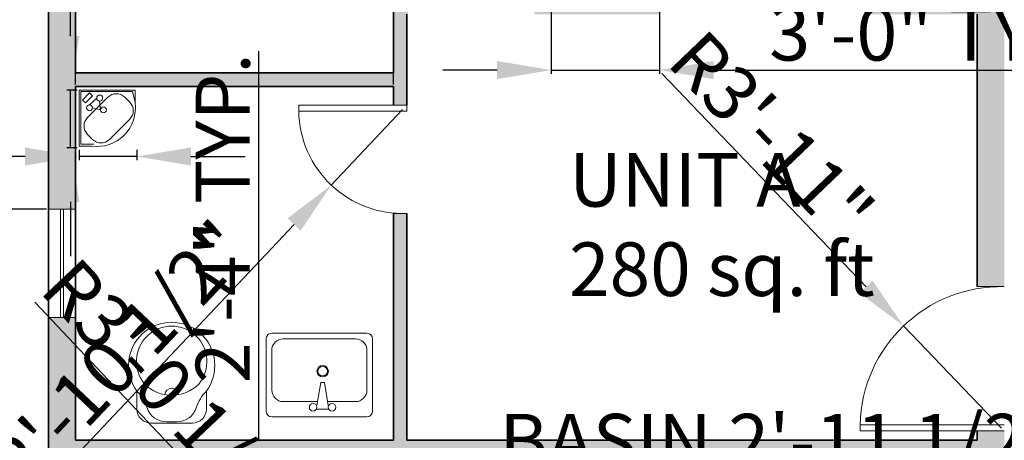
# Model space of a CAD drawing. Units: inches. Extents: x 2043 to 3177, y 1429 to 2563.
# Tile 10 of 14: x 2224 to 2552, y 1952 to 2092. Entities that reach past the tile are written whole.
import ezdxf

# ---------------------------------------------------------------- set-up
doc = ezdxf.new("R2010")
doc.units = ezdxf.units.IN
for name, color, linetype, lineweight in [('A-ANNO-DIMS', 2, 'Continuous', 13), ('A-AREA-IDEN', 7, 'Continuous', 18), ('A-DOOR', 3, 'Continuous', 18), ('A-FLOR-FIXT', 8, 'Continuous', 18), ('A-GLAZ', 4, 'Continuous', 18), ('A-WALL', 7, 'Continuous', 35)]:
    doc.layers.add(name, color=color, linetype=linetype, lineweight=lineweight)
doc.layers.add('A-WALL-PATT', color=251, linetype='Continuous', lineweight=13, true_color=0x636466)
doc.styles.add('DIM_FONT', font='TXT.shx', dxfattribs={"width": 0.8})
doc.styles.get("Standard").update_dxf_attribs({"font": 'arial.ttf'})
doc.dimstyles.new('ISO-25', dxfattribs={"dimtxt": 18, "dimasz": 18, "dimexe": 1.25, "dimexo": 0.625, "dimtad": 1, "dimlunit": 3, "dimtxsty": 'Standard', "dimcen": 2.5, "dimadec": 0, "dimazin": 0, "dimtfac": 1, "dimtmove": 0, "dimatfit": 3, "dimfxl": 1, "dimarcsym": 0})

# ---------------------------------------------------------------- blocks, each defined once
blk = doc.blocks.new('A$C6EF51710')
at = {"linetype": 'ByBlock'}
for p, q in [((0.0508, 0.2843), (0.1169, 0.2843)), ((0, 0.0811), (0, 0.2335)), ((0.0041, 0.1392), (0.0041, 0.1755)), ((0.1169, 0.0303), (0.0508, 0.0303))]:
    blk.add_line(p, q, dxfattribs=at)
for centre, radius, start, end in [((0.2107, 0.1573), 0.1576, 232.8984, 127.1016), ((0.0508, 0.2335), 0.0508, 90, 180), ((0.0168, 0.3818), 0.1397, 287.1046, 315), ((0.2413, 0.1573), 0.1397, 135, 225), ((0.2254, 0.1573), 0.1289, 230.0084, 129.9916), ((0.0803, 0.1755), 0.0762, 107.1046, 180), ((0.1016, 0.1573), 0.0254, 275.2159, 84.7841), ((0.0803, 0.1392), 0.0762, 180, 252.8954), ((0.0508, 0.0811), 0.0508, 180, 270), ((0.0168, -0.0672), 0.1397, 45, 72.8954)]:
    blk.add_arc(centre, radius, start, end, dxfattribs=at)
blk = doc.blocks.new('A$C03A44EBA')
at = {"rotation": 270}
blk.add_blockref('A$C6EF51710', (0.0003, 0.3683), dxfattribs=at)
blk = doc.blocks.new('A$C564A496C')
at = {"linetype": 'ByBlock'}
for p, q in [((543.2, 450), (30.7, 450)), ((0, 419.3), (0, 30.7)), ((238.5, 409.1), (299.8, 409.1)), ((238.5, 388.6), (258.9, 265.9)), ((279.4, 265.9), (299.8, 388.6)), ((573.8, 30.7), (573.8, 419.3)), ((92, 368.2), (243.6, 368.2)), ((294.7, 368.2), (481.8, 368.2)), ((30.7, 92), (30.7, 306.8)), ((258.9, 265.9), (279.4, 265.9)), ((543.2, 306.8), (543.2, 92)), ((30.7, 0), (543.2, 0)), ((481.8, 30.7), (92, 30.7))]:
    blk.add_line(p, q, dxfattribs=at)
for centre, radius in [((218, 398.9), 20.5), ((320.3, 398.9), 20.5), ((269.1, 204.5), 30.7), ((269.1, 204.5), 25.7)]:
    blk.add_circle(centre, radius, dxfattribs=at)
for centre, radius, start, end in [((30.7, 419.3), 30.7, 90, 180), ((543.2, 419.3), 30.7, 0, 90), ((92, 306.8), 61.4, 90, 180), ((481.8, 306.8), 61.4, 0, 90), ((92, 92), 61.4, 180, 270), ((481.8, 92), 61.4, 270, 0), ((30.7, 30.7), 30.7, 180, 270), ((543.2, 30.7), 30.7, 270, 0)]:
    blk.add_arc(centre, radius, start, end, dxfattribs=at)
at = {"style": 'DIM_FONT', "width": 0.8, "flags": 9}
for tag in ['YSIZE', 'XSIZE']:
    blk.add_attdef(tag, (269.1, 450), '', height=0.5, rotation=270, dxfattribs=at)
blk = doc.blocks.new('A$C017A17F4')
for p, q in [((0.45, 0.45), (0, 0.45)), ((0, 0.45), (0, 0.35)), ((0.3467, 0.3997), (0.3704, 0.4234)), ((0.4041, 0.3423), (0.3467, 0.3997)), ((0.3704, 0.4234), (0.4278, 0.366)), ((0.45, 0), (0.45, 0.45)), ((0.0533, 0.3414), (0.094, 0.3821)), ((0.2297, 0.3821), (0.3933, 0.2185)), ((0.4278, 0.366), (0.4041, 0.3423)), ((0.2168, 0.0421), (0.0533, 0.2056)), ((0.3933, 0.0827), (0.3526, 0.0421)), ((0.35, 0), (0.45, 0))]:
    blk.add_line(p, q)
at = {"ltscale": 10}
for p, q in [((0.4392, 0.4359), (0.0144, 0.4359)), ((0.0144, 0.4359), (0.0144, 0.3323)), ((0.4392, 0.4359), (0.4392, 0.0216)), ((0.3078, 0.342), (0.2911, 0.2778)), ((0.3317, 0.3659), (0.3861, 0.3086)), ((0.3622, 0.2847), (0.2911, 0.2778)), ((0.4392, 0.0216), (0.35, 0))]:
    blk.add_line(p, q, dxfattribs=at)
for centre in [(0.3078, 0.3659), (0.2911, 0.2539), (0.3861, 0.2847)]:
    blk.add_circle(centre, 0.0239, dxfattribs=at)
for centre, radius, start, end in [((0.1618, 0.3142), 0.096, 45, 135), ((0.3045, 0.3045), 0.3079, 171.50989, 278.49011), ((0.1212, 0.2735), 0.096, 135, 225), ((0.3254, 0.1506), 0.096, 315, 45), ((0.2847, 0.11), 0.096, 225, 315)]:
    blk.add_arc(centre, radius, start, end)
blk = doc.blocks.new('*D26')
at = {"layer": 'A-ANNO-DIMS', "color": 0, "lineweight": -2, "transparency": 16777216}
for p, q in [((2233.12, 2029.27), (2166.79, 2029.27)), ((2168.04, 1902.52), (2168.04, 2011.27)), ((2233.12, 1884.52), (2166.79, 1884.52))]:
    blk.add_line(p, q, dxfattribs=at)
at = {"layer": 'A-ANNO-DIMS', "color": 0, "transparency": 16777216}
for points in [[(2165.04, 2011.27), (2171.04, 2011.27), (2168.04, 2029.27)], [(2165.04, 1902.52), (2171.04, 1902.52), (2168.04, 1884.52)]]:
    blk.add_solid(points, dxfattribs=at)
at = {"layer": 'Defpoints', "color": 0, "transparency": 16777216}
for p in [(2168.04, 2029.27), (2233.74, 2029.27), (2233.74, 1884.52)]:
    blk.add_point(p, dxfattribs=at)
at = {"layer": 'A-ANNO-DIMS', "color": 0, "transparency": 16777216, "insert": (2158.23, 1956.89), "char_height": 18, "attachment_point": 5, "rotation": 90}
blk.add_mtext('19\'-0"', dxfattribs=at)
blk = doc.blocks.new('*D27')
at = {"layer": 'A-ANNO-DIMS', "color": 0, "lineweight": -2, "transparency": 16777216}
for p, q in [((2233.12, 2261.39), (2165.87, 2261.39)), ((2167.12, 2047.27), (2167.12, 2243.39)), ((2233.12, 2029.27), (2165.87, 2029.27))]:
    blk.add_line(p, q, dxfattribs=at)
at = {"layer": 'A-ANNO-DIMS', "color": 0, "transparency": 16777216}
for points in [[(2164.12, 2243.39), (2170.12, 2243.39), (2167.12, 2261.39)], [(2164.12, 2047.27), (2170.12, 2047.27), (2167.12, 2029.27)]]:
    blk.add_solid(points, dxfattribs=at)
at = {"layer": 'Defpoints', "color": 0, "transparency": 16777216}
for p in [(2167.12, 2261.39), (2233.74, 2261.39), (2233.74, 2029.27)]:
    blk.add_point(p, dxfattribs=at)
at = {"layer": 'A-ANNO-DIMS', "color": 0, "transparency": 16777216, "insert": (2157.3, 2145.33), "char_height": 18, "attachment_point": 5, "rotation": 90}
blk.add_mtext('25\'-0"', dxfattribs=at)
blk = doc.blocks.new('*D28')
at = {"layer": 'A-ANNO-DIMS', "color": 0, "lineweight": -2, "transparency": 16777216}
for p, q in [((2233.12, 2261.39), (2064.1, 2261.39)), ((2065.35, 2243.39), (2065.35, 1652.39)), ((2233.12, 1634.39), (2064.1, 1634.39))]:
    blk.add_line(p, q, dxfattribs=at)
at = {"layer": 'A-ANNO-DIMS', "color": 0, "transparency": 16777216}
for points in [[(2062.35, 2243.39), (2068.35, 2243.39), (2065.35, 2261.39)], [(2062.35, 1652.39), (2068.35, 1652.39), (2065.35, 1634.39)]]:
    blk.add_solid(points, dxfattribs=at)
at = {"layer": 'Defpoints', "color": 0, "transparency": 16777216}
for p in [(2233.74, 2261.39), (2065.35, 1634.39), (2233.74, 1634.39)]:
    blk.add_point(p, dxfattribs=at)
at = {"layer": 'A-ANNO-DIMS', "color": 0, "transparency": 16777216, "insert": (2055.54, 1947.89), "char_height": 18, "attachment_point": 5, "rotation": 90}
blk.add_mtext('75\'-0"', dxfattribs=at)
blk = doc.blocks.new('GLAZING-36')
for p, q in [((0, 36), (0, 0)), ((1, 36), (1, 0))]:
    blk.add_line(p, q)
blk = doc.blocks.new('*D57')
at = {"layer": 'A-ANNO-DIMS', "color": 0, "lineweight": -2, "transparency": 16777216}
for p, q in [((2291.03, 1939.93), (2273.03, 1939.93)), ((2309.03, 1935.24), (2309.03, 1941.18)), ((2309.03, 1939.93), (2344.46, 1939.93)), ((2344.46, 1935.24), (2344.46, 1941.18)), ((2362.46, 1939.93), (2629.01, 1939.93))]:
    blk.add_line(p, q, dxfattribs=at)
at = {"layer": 'A-ANNO-DIMS', "color": 0, "transparency": 16777216}
for points in [[(2291.03, 1942.93), (2291.03, 1936.93), (2309.03, 1939.93)], [(2362.46, 1942.93), (2362.46, 1936.93), (2344.46, 1939.93)]]:
    blk.add_solid(points, dxfattribs=at)
at = {"layer": 'Defpoints', "color": 0, "transparency": 16777216}
for p in [(2344.46, 1939.93), (2309.03, 1934.62), (2344.46, 1934.62)]:
    blk.add_point(p, dxfattribs=at)
at = {"layer": 'A-ANNO-DIMS', "color": 0, "transparency": 16777216, "insert": (2504.74, 1949.86), "char_height": 18, "attachment_point": 5}
blk.add_mtext('BASIN 2\'-11 1/2" TYP.', dxfattribs=at)
blk = doc.blocks.new('*D58')
at = {"layer": 'A-ANNO-DIMS', "color": 0, "lineweight": -2, "transparency": 16777216}
for p, q in [((2303.72, 1952.62), (2303.72, 2081.89)), ((2308.41, 1934.62), (2302.47, 1934.62)), ((2303.72, 1906.83), (2303.72, 1934.62)), ((2308.41, 1906.83), (2302.47, 1906.83)), ((2303.72, 1888.83), (2303.72, 1870.83))]:
    blk.add_line(p, q, dxfattribs=at)
at = {"layer": 'A-ANNO-DIMS', "color": 0, "transparency": 16777216}
for points in [[(2300.72, 1952.62), (2306.72, 1952.62), (2303.72, 1934.62)], [(2300.72, 1888.83), (2306.72, 1888.83), (2303.72, 1906.83)]]:
    blk.add_solid(points, dxfattribs=at)
at = {"layer": 'Defpoints', "color": 0, "transparency": 16777216}
for p in [(2303.72, 1934.62), (2309.03, 1934.62), (2309.03, 1906.83)]:
    blk.add_point(p, dxfattribs=at)
at = {"layer": 'A-ANNO-DIMS', "color": 0, "transparency": 16777216, "insert": (2294.05, 2026.26), "char_height": 18, "attachment_point": 5, "rotation": 90}
blk.add_mtext('2\'-4" TYP.', dxfattribs=at)
blk = doc.blocks.new('*D59')
at = {"layer": 'A-ANNO-DIMS', "color": 0, "lineweight": -2, "transparency": 16777216}
for p, q in [((2241.04, 2086.9), (2241.04, 2414.07)), ((2243.29, 2068.9), (2239.79, 2068.9)), ((2241.04, 2049.7), (2241.04, 2068.9)), ((2243.29, 2049.7), (2239.79, 2049.7)), ((2241.04, 2031.7), (2241.04, 2013.7))]:
    blk.add_line(p, q, dxfattribs=at)
at = {"layer": 'A-ANNO-DIMS', "color": 0, "transparency": 16777216}
for points in [[(2238.04, 2086.9), (2244.04, 2086.9), (2241.04, 2068.9)], [(2238.04, 2031.7), (2244.04, 2031.7), (2241.04, 2049.7)]]:
    blk.add_solid(points, dxfattribs=at)
at = {"layer": 'Defpoints', "color": 0, "transparency": 16777216}
for p in [(2241.04, 2068.9), (2243.92, 2068.9), (2243.92, 2049.7)]:
    blk.add_point(p, dxfattribs=at)
at = {"layer": 'A-ANNO-DIMS', "color": 0, "transparency": 16777216, "insert": (2231.1, 2259.48), "char_height": 18, "attachment_point": 5, "rotation": 90}
blk.add_mtext('CORNER BASIN 1\'-7" TYP.', dxfattribs=at)
blk = doc.blocks.new('*D60')
at = {"layer": 'A-ANNO-DIMS', "color": 0, "lineweight": -2, "transparency": 16777216}
for p, q in [((2243.92, 2049.08), (2243.92, 2045.57)), ((2263.12, 2049.08), (2263.12, 2045.57)), ((2225.92, 2046.82), (2098.64, 2046.82)), ((2263.12, 2046.82), (2243.92, 2046.82)), ((2281.12, 2046.82), (2299.12, 2046.82))]:
    blk.add_line(p, q, dxfattribs=at)
at = {"layer": 'A-ANNO-DIMS', "color": 0, "transparency": 16777216}
for points in [[(2225.92, 2049.82), (2225.92, 2043.82), (2243.92, 2046.82)], [(2281.12, 2049.82), (2281.12, 2043.82), (2263.12, 2046.82)]]:
    blk.add_solid(points, dxfattribs=at)
at = {"layer": 'Defpoints', "color": 0, "transparency": 16777216}
for p in [(2243.92, 2049.7), (2263.12, 2049.7), (2243.92, 2046.82)]:
    blk.add_point(p, dxfattribs=at)
at = {"layer": 'A-ANNO-DIMS', "color": 0, "transparency": 16777216, "insert": (2153.28, 2056.49), "char_height": 18, "attachment_point": 5}
blk.add_mtext('1\'-7" TYP.', dxfattribs=at)
blk = doc.blocks.new('*D61')
at = {"layer": 'A-ANNO-DIMS', "color": 0, "lineweight": -2, "transparency": 16777216}
for p, q in [((2752.39, 1913.46), (2434.98, 1913.46)), ((2770.39, 1916.38), (2770.39, 1912.21)), ((2794.01, 1913.46), (2770.39, 1913.46)), ((2794.01, 1916.38), (2794.01, 1912.21)), ((2812.01, 1913.46), (2830.01, 1913.46))]:
    blk.add_line(p, q, dxfattribs=at)
at = {"layer": 'A-ANNO-DIMS', "color": 0, "transparency": 16777216}
for points in [[(2752.39, 1916.46), (2752.39, 1910.46), (2770.39, 1913.46)], [(2812.01, 1916.46), (2812.01, 1910.46), (2794.01, 1913.46)]]:
    blk.add_solid(points, dxfattribs=at)
at = {"layer": 'Defpoints', "color": 0, "transparency": 16777216}
for p in [(2770.39, 1917.01), (2794.01, 1917.01), (2770.39, 1913.46)]:
    blk.add_point(p, dxfattribs=at)
at = {"layer": 'A-ANNO-DIMS', "color": 0, "transparency": 16777216, "insert": (2584.68, 1923.4), "char_height": 18, "attachment_point": 5}
blk.add_mtext('COOKTOP 1\'-11 1/2" TYP.', dxfattribs=at)
blk = doc.blocks.new('*D64')
at = {"layer": 'A-ANNO-DIMS', "color": 0, "lineweight": -2, "transparency": 16777216}
for p, q in [((2400.99, 2098.02), (2400.99, 2074.33)), ((2436.99, 2098.02), (2436.99, 2074.33)), ((2382.99, 2075.58), (2364.99, 2075.58)), ((2400.99, 2075.58), (2436.99, 2075.58)), ((2454.99, 2075.58), (2583.95, 2075.58))]:
    blk.add_line(p, q, dxfattribs=at)
at = {"layer": 'A-ANNO-DIMS', "color": 0, "transparency": 16777216}
for points in [[(2382.99, 2078.58), (2382.99, 2072.58), (2400.99, 2075.58)], [(2454.99, 2078.58), (2454.99, 2072.58), (2436.99, 2075.58)]]:
    blk.add_solid(points, dxfattribs=at)
at = {"layer": 'Defpoints', "color": 0, "transparency": 16777216}
for p in [(2400.99, 2098.64), (2436.99, 2098.64), (2436.99, 2075.58)]:
    blk.add_point(p, dxfattribs=at)
at = {"layer": 'A-ANNO-DIMS', "color": 0, "transparency": 16777216, "insert": (2528.47, 2085.4), "char_height": 18, "attachment_point": 5}
blk.add_mtext('3\'-0" TYP.', dxfattribs=at)
blk = doc.blocks.new('*D73')
at = {"layer": 'A-ANNO-DIMS', "color": 0, "lineweight": -2, "transparency": 16777216}
for p, q in [((2242.74, 2070.77), (2242.74, 2125.49)), ((2260.74, 2124.24), (2330.49, 2124.24)), ((2348.49, 2070.77), (2348.49, 2125.49))]:
    blk.add_line(p, q, dxfattribs=at)
at = {"layer": 'A-ANNO-DIMS', "color": 0, "transparency": 16777216}
for points in [[(2260.74, 2127.24), (2260.74, 2121.24), (2242.74, 2124.24)], [(2330.49, 2127.24), (2330.49, 2121.24), (2348.49, 2124.24)]]:
    blk.add_solid(points, dxfattribs=at)
at = {"layer": 'Defpoints', "color": 0, "transparency": 16777216}
for p in [(2348.49, 2124.24), (2242.74, 2070.14), (2348.49, 2070.14)]:
    blk.add_point(p, dxfattribs=at)
at = {"layer": 'A-ANNO-DIMS', "color": 0, "transparency": 16777216, "insert": (2295.62, 2134.06), "char_height": 18, "attachment_point": 5}
blk.add_mtext('8\'-10"', dxfattribs=at)
blk = doc.blocks.new('*D83')
at = {"layer": 'A-ANNO-DIMS', "color": 0, "lineweight": -2, "transparency": 16777216}
for p, q in [((2437.75, 2074.42), (2505.77, 2003.44)), ((2550.78, 1956.48), (2518.23, 1990.44))]:
    blk.add_line(p, q, dxfattribs=at)
at = {"layer": 'A-ANNO-DIMS', "color": 0, "transparency": 16777216}
blk.add_solid([(2507.94, 2005.52), (2503.61, 2001.36), (2518.23, 1990.44)], dxfattribs=at)
at = {"layer": 'Defpoints', "color": 0, "transparency": 16777216}
for p in [(2518.23, 1990.44), (2550.78, 1956.48)]:
    blk.add_point(p, dxfattribs=at)
at = {"layer": 'A-ANNO-DIMS', "color": 0, "transparency": 16777216, "insert": (2472.63, 2052.22), "char_height": 18, "attachment_point": 5, "rotation": 313.7813}
blk.add_mtext('R3\'-11"', dxfattribs=at)
blk = doc.blocks.new('*D91')
at = {"layer": 'A-ANNO-DIMS', "color": 0, "lineweight": -2, "transparency": 16777216}
for p, q in [((2229.24, 1998.38), (2315.93, 1906.58)), ((2353.2, 1867.12), (2328.29, 1893.49))]:
    blk.add_line(p, q, dxfattribs=at)
at = {"layer": 'A-ANNO-DIMS', "color": 0, "transparency": 16777216}
blk.add_solid([(2318.11, 1908.64), (2313.75, 1904.52), (2328.29, 1893.49)], dxfattribs=at)
at = {"layer": 'Defpoints', "color": 0, "transparency": 16777216}
for p in [(2328.29, 1893.49), (2353.2, 1867.12)]:
    blk.add_point(p, dxfattribs=at)
at = {"layer": 'A-ANNO-DIMS', "color": 0, "transparency": 16777216, "insert": (2273.63, 1965.84), "char_height": 18, "attachment_point": 5, "rotation": 313.3628}
blk.add_mtext('R3\'-0 1/2"', dxfattribs=at)
blk = doc.blocks.new('*D92')
at = {"layer": 'A-ANNO-DIMS', "color": 0, "lineweight": -2, "transparency": 16777216}
for p, q in [((2351.56, 2062.42), (2327.82, 2037.29)), ((2219.16, 1922.24), (2315.46, 2024.21))]:
    blk.add_line(p, q, dxfattribs=at)
at = {"layer": 'A-ANNO-DIMS', "color": 0, "transparency": 16777216}
blk.add_solid([(2313.28, 2026.27), (2317.64, 2022.15), (2327.82, 2037.29)], dxfattribs=at)
at = {"layer": 'Defpoints', "color": 0, "transparency": 16777216}
for p in [(2351.56, 2062.42), (2327.82, 2037.29)]:
    blk.add_point(p, dxfattribs=at)
at = {"layer": 'A-ANNO-DIMS', "color": 0, "transparency": 16777216, "insert": (2253.91, 1973.5), "char_height": 18, "attachment_point": 5, "rotation": 46.6358}
blk.add_mtext('R2\'-10 1/2"', dxfattribs=at)

msp = doc.modelspace()

# ---------------------------------------------------------------- hatches: boundary and pattern name
at = {"layer": 'A-WALL-PATT'}
h = msp.add_hatch(color=256, dxfattribs=at)
h.dxf.hatch_style = 1
h.paths.add_polyline_path([(2283.62, 2261.393), (2233.745, 2261.393), (2233.745, 2029.268), (2242.745, 2029.268), (2242.745, 2070.143), (2348.495, 2070.143), (2348.495, 2063.887), (2352.995, 2063.887), (2352.995, 2094.143), (2353.364, 2094.143, -0.017175), (2353.364, 2096.932), (2353.364, 2098.643), (2348.495, 2098.643), (2348.495, 2096.393), (2348.495, 2074.643), (2242.745, 2074.643), (2242.745, 2252.393), (2283.62, 2252.393)])
h.paths.add_polyline_path([(2453.87, 2261.393), (2355.62, 2261.393), (2355.62, 2252.393), (2396.495, 2252.393), (2396.495, 2098.643), (2395.364, 2098.643), (2395.364, 2094.143), (2436.995, 2094.143), (2436.995, 2098.643), (2400.995, 2098.643), (2400.995, 2252.393), (2453.87, 2252.393)])
h.paths.add_polyline_path([(2551.745, 2261.393), (2489.87, 2261.393), (2489.87, 2252.393), (2542.745, 2252.393), (2542.745, 2098.643), (2506.745, 2098.643), (2506.745, 2094.143), (2542.745, 2094.143), (2542.745, 2003.513), (2549.809, 2003.513, -0.0102854), (2551.745, 2003.513), (2551.745, 2195.393), (2571.245, 2195.393), (2571.245, 2204.393), (2551.745, 2204.393)])
h.paths.add_polyline_path([(2724.62, 2261.393), (2662.745, 2261.393), (2662.745, 2204.393), (2643.245, 2204.393), (2643.245, 2195.393), (2662.745, 2195.393), (2662.745, 2002.566, -0.0156152), (2665.651, 2002.566), (2671.745, 2002.566), (2671.745, 2094.143), (2707.745, 2094.143), (2707.745, 2098.643), (2671.745, 2098.643), (2671.745, 2252.393), (2724.62, 2252.393)])
h.paths.add_polyline_path([(2858.87, 2261.393), (2760.62, 2261.393), (2760.62, 2252.393), (2813.495, 2252.393), (2813.495, 2098.643), (2777.495, 2098.643), (2777.495, 2094.143), (2819.302, 2094.143), (2819.302, 2098.643), (2817.995, 2098.643), (2817.995, 2252.393), (2858.87, 2252.393)])
h.paths.add_polyline_path([(2980.745, 2261.393), (2930.87, 2261.393), (2930.87, 2252.393), (2971.745, 2252.393), (2971.745, 2074.643), (2865.995, 2074.643), (2865.995, 2098.643), (2861.429, 2098.643, -0.0279128), (2861.495, 2094.143), (2861.495, 2063.254), (2865.995, 2063.254), (2865.995, 2070.143), (2971.745, 2070.143), (2971.745, 2029.268), (2980.745, 2029.268)])
h.paths.add_polyline_path([(2980.745, 1993.268), (2971.745, 1993.268), (2971.745, 1952.393), (2865.995, 1952.393), (2865.995, 2027.254), (2865.688, 2027.254, -0.0309542), (2861.495, 2027.254), (2861.495, 1952.393), (2671.745, 1952.393), (2671.745, 1954.566), (2662.745, 1954.566), (2662.745, 1883.393), (2661.473, 1883.393, -0.012912), (2661.473, 1880.977), (2661.473, 1874.393), (2671.745, 1874.393), (2671.745, 1943.393), (2861.495, 1943.393), (2861.495, 1903.412, -0.0351753), (2865.995, 1903.659), (2865.995, 1943.393), (2971.745, 1943.393), (2971.745, 1922.018), (2980.745, 1922.018)])
h.paths.add_polyline_path([(2980.745, 1886.018), (2971.745, 1886.018), (2971.745, 1864.643), (2865.995, 1864.643), (2865.995, 1867.412), (2861.495, 1867.412), (2861.495, 1840.643), (2828.844, 1840.643, -0.0159075), (2828.844, 1837.684), (2828.844, 1836.143), (2865.995, 1836.143), (2865.995, 1860.143), (2971.745, 1860.143), (2971.745, 1643.393), (2910.245, 1643.393), (2910.245, 1634.393), (2980.745, 1634.393)])
h.paths.add_polyline_path([(2776.745, 1836.143), (2780.844, 1836.143), (2780.844, 1840.643), (2772.245, 1840.643), (2772.245, 1679.393), (2760.995, 1679.393), (2760.995, 1670.393), (2767.745, 1670.393), (2767.745, 1634.393), (2838.245, 1634.393), (2838.245, 1643.393), (2776.745, 1643.393)])
h.paths.add_polyline_path([(2736.995, 1679.393), (2727.995, 1679.393), (2727.995, 1670.393), (2736.995, 1670.393)])
h.paths.add_polyline_path([(2667.995, 1679.393), (2611.745, 1679.393), (2611.745, 1874.393), (2613.473, 1874.393), (2613.473, 1883.393), (2600.336, 1883.393), (2600.336, 1874.393), (2602.745, 1874.393), (2602.745, 1679.393), (2546.495, 1679.393), (2546.495, 1670.393), (2667.995, 1670.393)])
h.paths.add_polyline_path([(2486.495, 1679.393), (2477.495, 1679.393), (2477.495, 1670.393), (2486.495, 1670.393)])
h.paths.add_polyline_path([(2453.495, 1679.393), (2442.245, 1679.393), (2442.245, 1839.893), (2427.654, 1839.893), (2427.654, 1835.393), (2437.745, 1835.393), (2437.745, 1643.393), (2376.245, 1643.393), (2376.245, 1634.393), (2446.745, 1634.393), (2446.745, 1670.393), (2453.495, 1670.393)])
h.paths.add_polyline_path([(2304.245, 1643.393), (2242.745, 1643.393), (2242.745, 1857.143), (2348.495, 1857.143), (2348.495, 1835.393), (2352.995, 1835.393), (2379.654, 1835.393), (2379.654, 1837.073, -0.0151369), (2379.654, 1839.893), (2352.995, 1839.893), (2352.995, 1867.394), (2348.495, 1867.394), (2348.495, 1861.643), (2242.745, 1861.643), (2242.745, 1884.518), (2233.745, 1884.518), (2233.745, 1634.393), (2304.245, 1634.393)])
h.paths.add_polyline_path([(2551.745, 1955.513), (2542.745, 1955.513), (2542.745, 1952.393), (2352.995, 1952.393), (2352.995, 2027.887, -0.0208198), (2350.117, 2027.887), (2348.495, 2027.887), (2348.495, 1952.393), (2242.745, 1952.393), (2242.745, 1993.268), (2233.745, 1993.268), (2233.745, 1943.393), (2233.745, 1920.518), (2242.745, 1920.518), (2242.745, 1943.393), (2348.495, 1943.393), (2348.495, 1903.394), (2352.995, 1903.394), (2352.995, 1943.393), (2542.745, 1943.393), (2542.745, 1874.393), (2552.336, 1874.393), (2552.336, 1880.494, -0.0155728), (2552.336, 1883.393), (2551.745, 1883.393)])

# ---------------------------------------------------------------- linework, layer by layer
at = {"layer": 'A-DOOR'}
for p, q in [((2352.995, 2063.887), (2316.995, 2063.887)), ((2316.995, 2063.887), (2316.995, 2061.887)), ((2348.495, 2063.887), (2352.995, 2063.887)), ((2352.995, 2061.887), (2352.995, 2063.887)), ((2316.995, 2061.887), (2352.995, 2061.887)), ((2348.495, 2027.887), (2352.995, 2027.887)), ((2542.745, 2003.513), (2551.745, 2003.513)), ((2503.745, 1955.513), (2503.745, 1957.513)), ((2503.745, 1957.513), (2551.745, 1957.513)), ((2551.745, 1955.513), (2503.745, 1955.513)), ((2542.745, 1955.513), (2551.745, 1955.513))]:
    msp.add_line(p, q, dxfattribs=at)
for centre, radius, start, end in [((2351.556, 2062.422), 34.565, 180.88773, 272.38543), ((2550.777, 1956.479), 47.044, 88.82142, 178.74083)]:
    msp.add_arc(centre, radius, start, end, dxfattribs=at)
at = {"layer": 'A-GLAZ'}
for p, q in [((2242.745, 2029.268), (2233.745, 2029.268)), ((2242.745, 1993.268), (2233.745, 1993.268))]:
    msp.add_line(p, q, dxfattribs=at)
at = {"layer": 'A-WALL'}
for p, q in [((2233.745, 2261.393), (2233.745, 1943.393)), ((2242.745, 2252.393), (2242.745, 2074.643)), ((2348.495, 2096.393), (2348.495, 2074.643)), ((2352.995, 2094.143), (2352.995, 2063.887)), ((2542.745, 2094.143), (2542.745, 2003.513)), ((2242.745, 2074.643), (2348.495, 2074.643)), ((2242.745, 2070.143), (2348.495, 2070.143)), ((2242.745, 2070.143), (2242.745, 1952.393)), ((2348.495, 2070.143), (2348.495, 2063.887)), ((2348.495, 2027.887), (2348.495, 1952.393)), ((2352.995, 2027.887), (2352.995, 1952.393)), ((2542.745, 1955.513), (2542.745, 1952.393)), ((2242.745, 1952.393), (2348.495, 1952.393)), ((2352.995, 1952.393), (2542.745, 1952.393))]:
    msp.add_line(p, q, dxfattribs=at)

# ---------------------------------------------------------------- block references
at = {"layer": 'A-FLOR-FIXT'}
for name, p, xscale, yscale, zscale, rotation in [('A$C017A17F4', (2262.523, 2050.298), 41.3428040046008, 41.3428040046008, 41.3428040046008, 90), ('A$C03A44EBA', (2289.057, 1991.649), 91.00031060141868, 91.00031060141868, 91.00031060141868, 180), ('A$C564A496C', (2341.561, 1988.003), 0.0617427035267454, 0.0617427035267454, 0.0617427035267454, 180)]:
    msp.add_blockref(name, p, dxfattribs=dict(at, xscale=xscale, yscale=yscale, zscale=zscale, rotation=rotation))
at = {"layer": 'A-GLAZ'}
msp.add_blockref('GLAZING-36', (2237.745, 1993.268), dxfattribs=at)

# ---------------------------------------------------------------- texts
at = {"layer": 'A-AREA-IDEN', "insert": (2406.914, 2047.961), "char_height": 17.8269, "attachment_point": 1}
msp.add_mtext_dynamic_manual_height_columns('UNIT A \\P280 sq. ft', width=505.18079, gutter_width=89.135, heights=[0], dxfattribs=at)

# ---------------------------------------------------------------- dimensions: what is measured, and where the dimension line sits
at = {"layer": 'A-ANNO-DIMS'}
for base, p1, p2, angle, text, override, picture, middle in [((2241.039, 2068.902), (2243.919, 2049.702), (2243.919, 2068.902), 90, 'CORNER BASIN <> TYP.', {"dimdec": 1, "dimlfac": 1, "dimrnd": 0, "dimzin": 1, "dimdsep": 46, "dimlunit": 4, "dimfrac": 2}, '*D59', (2231.101, 2259.485)), ((2065.352, 1634.393), (2233.745, 2261.393), (2233.745, 1634.393), 90, '75\'-0"', {"dimclrd": 0, "dimclre": 0, "dimclrt": 0}, '*D28', (2055.537, 1947.893)), ((2167.117, 2261.393), (2233.745, 2029.268), (2233.745, 2261.393), 90, '25\'-0"', {"dimclrd": 0, "dimclre": 0, "dimclrt": 0}, '*D27', (2157.302, 2145.331)), ((2243.919, 2046.822), (2263.119, 2049.702), (2243.919, 2049.702), 180, '<> TYP.', {"dimdec": 1, "dimlfac": 1, "dimrnd": 0, "dimzin": 1, "dimdsep": 46, "dimlunit": 4, "dimfrac": 2}, '*D60', (2153.282, 2056.49)), ((2303.717, 1934.617), (2309.031, 1906.833), (2309.031, 1934.617), 90, '<> TYP.', {"dimdec": 1, "dimlfac": 1, "dimrnd": 0, "dimzin": 1, "dimdsep": 46, "dimlunit": 4, "dimfrac": 2}, '*D58', (2294.049, 2026.255)), ((2168.041, 2029.268), (2233.745, 1884.518), (2233.745, 2029.268), 90, '19\'-0"', {"dimclrd": 0, "dimclre": 0, "dimclrt": 0}, '*D26', (2158.225, 1956.893)), ((2770.393, 1913.464), (2794.015, 1917.007), (2770.393, 1917.007), 180, 'COOKTOP <> TYP.', {"dimdec": 1, "dimlfac": 1, "dimrnd": 0, "dimzin": 1, "dimdsep": 46, "dimlunit": 4, "dimfrac": 2}, '*D61', (2584.685, 1923.402))]:
    dim = msp.add_linear_dim(base=base, p1=p1, p2=p2, angle=angle, text=text, dimstyle='ISO-25', override=override, dxfattribs=at)
    dim.commit()
    dim.dimension.update_dxf_attribs({"geometry": picture, "text_midpoint": middle})
dim = msp.add_linear_dim(base=(2348.494581, 2124.243329), p1=(2242.744581, 2070.143329), p2=(2348.494581, 2070.143329), dimstyle='ISO-25', override={"dimdec": 1, "dimlfac": 1, "dimrnd": 0, "dimzin": 1, "dimdsep": 46, "dimlunit": 4, "dimfrac": 2}, dxfattribs=at)
dim.commit()
dim.dimension.update_dxf_attribs({"geometry": '*D73', "text_midpoint": (2295.619581, 2134.058642779)})
for base, p1, p2, text, picture, middle in [((2436.995, 2075.581), (2400.995, 2098.643), (2436.995, 2098.643), '<> TYP.', '*D64', (2528.473, 2085.402)), ((2344.462, 1939.932), (2309.031, 1934.617), (2344.462, 1934.617), 'BASIN <> TYP.', '*D57', (2504.735, 1949.864))]:
    dim = msp.add_linear_dim(base=base, p1=p1, p2=p2, text=text, dimstyle='ISO-25', override={"dimdec": 1, "dimlfac": 1, "dimrnd": 0, "dimzin": 1, "dimdsep": 46, "dimlunit": 4, "dimfrac": 2}, dxfattribs=at)
    dim.commit()
    dim.dimension.update_dxf_attribs({"geometry": picture, "text_midpoint": middle})
for center, mpoint, picture, middle in [((2550.777, 1956.479), (2518.227, 1990.444), '*D83', (2472.626, 2052.222)), ((2351.556, 2062.422), (2327.822, 2037.293), '*D92', (2253.911, 1973.501)), ((2353.201, 1867.116), (2328.292, 1893.491), '*D91', (2273.63, 1965.844))]:
    dim = msp.add_radius_dim(center=center, mpoint=mpoint, dimstyle='ISO-25', override={"dimdec": 1, "dimlfac": 1, "dimrnd": 0, "dimzin": 1, "dimdsep": 46, "dimlunit": 4, "dimfrac": 2}, dxfattribs=at)
    dim.commit()
    dim.dimension.update_dxf_attribs({"geometry": picture, "text_midpoint": middle})

doc.saveas('drawing.dxf')
